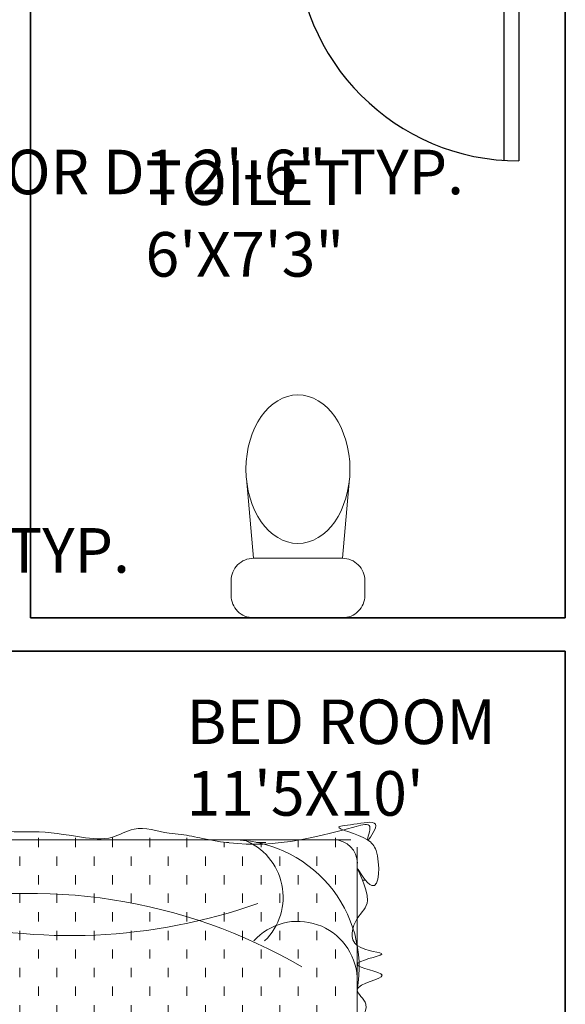
# Model space of a CAD drawing. Units: inches. Extents: x -26 to 575, y -18 to 513.
# Tile 9 of 28: x 196 to 269, y 191 to 324. Entities that reach past the tile are written whole.
import ezdxf

# ---------------------------------------------------------------- set-up
doc = ezdxf.new("R2010")
doc.units = ezdxf.units.IN
doc.header["$MEASUREMENT"] = 0
for name, color, linetype, lineweight in [('A-ANNO-DIMS', 2, 'Continuous', 18), ('A-AREA-IDEN', 7, 'Continuous', 18), ('A-DOOR', 3, 'Continuous', 25), ('A-FLOR-FIXT', 9, 'Continuous', 18), ('A-WALL', 7, 'Continuous', 35), ('Furniture', 8, 'Continuous', 15)]:
    doc.layers.add(name, color=color, linetype=linetype, lineweight=lineweight)
doc.styles.get("Standard").update_dxf_attribs({"font": 'arial.ttf', "height": 6})
doc.dimstyles.get("Standard").update_dxf_attribs({"dimtxt": 6, "dimasz": 0.18, "dimexe": 0.18, "dimexo": 0.0625, "dimgap": 0.09, "dimtad": 0, "dimtih": 1, "dimtoh": 1, "dimzin": 0, "dimdsep": 46, "dimlunit": 3, "dimtxsty": 'Standard', "dimcen": 0.09, "dimadec": 0, "dimazin": 0, "dimtfac": 1, "dimtofl": 0, "dimtmove": 0, "dimatfit": 3, "dimfxl": 1, "dimtolj": 1, "dimtzin": 0, "dimarcsym": 0})

# ---------------------------------------------------------------- blocks, each defined once
blk = doc.blocks.new('BED-DOUBLE-WITH-NIGHTSTANDS')
for p, q in [((1.93, 83.36), (1.93, 62.76)), ((21.61, 63.03), (21.61, 82.46)), ((22.83, 60.83), (22.83, 82.62)), ((81.88, 82.34), (81.88, 56.23)), ((82.67, 83.36), (82.67, 62.76)), ((102.35, 63.03), (102.35, 82.46)), ((23.23, 81.08), (0, 81.08)), ((10.27, 81.76), (8.94, 70.83)), ((21.24, 81.17), (81.88, 81.17)), ((103.97, 81.08), (80.74, 81.08)), ((20.89, 80.15), (2.67, 80.15)), ((2.67, 80.15), (2.67, 64.97)), ((20.89, 64.97), (20.89, 80.15)), ((82.67, 79.72), (21.06, 79.72)), ((101.63, 80.15), (83.41, 80.15)), ((83.41, 80.15), (83.41, 64.97)), ((101.63, 64.97), (101.63, 80.15)), ((92.57, 79.4), (92.57, 67.51)), ((14.67, 76.01), (4.51, 77.26)), ((44, 76.51), (44, 76.88)), ((46.83, 76.51), (46.83, 76.88)), ((8.06, 67.24), (12.03, 75.72)), ((12.03, 75.72), (14.23, 74.69)), ((25.06, 76.76), (22.83, 76.76)), ((41.17, 76.51), (40.96, 76.72)), ((41.17, 76.51), (41.43, 76.77)), ((41.17, 76.51), (41.17, 76.74)), ((56.23, 76.76), (41.36, 76.76)), ((44, 76.51), (43.73, 76.77)), ((44, 76.51), (44.26, 76.77)), ((46.83, 76.51), (46.56, 76.77)), ((46.83, 76.51), (47.09, 76.77)), ((57, 76.51), (56.74, 76.77)), ((57, 76.51), (57, 76.83)), ((57, 76.51), (57.27, 76.77)), ((81.88, 76.76), (59.39, 76.76)), ((59.83, 76.51), (59.59, 76.74)), ((59.83, 76.51), (59.83, 76.72)), ((59.83, 76.51), (60.02, 76.69)), ((11.46, 75.32), (8.12, 68.2)), ((14.23, 74.69), (10.26, 66.21)), ((11.77, 75.18), (11.46, 75.32)), ((25.61, 75.09), (25.35, 75.36)), ((25.61, 75.09), (25.61, 75.47)), ((25.61, 75.09), (25.88, 75.36)), ((28.44, 75.09), (28.18, 75.36)), ((28.44, 75.09), (28.44, 75.47)), ((28.44, 75.09), (28.71, 75.36)), ((31.27, 75.09), (31, 75.36)), ((31.27, 75.09), (31.27, 75.47)), ((31.27, 75.09), (31.53, 75.36)), ((34.1, 75.09), (33.83, 75.36)), ((34.1, 75.09), (34.1, 75.47)), ((34.1, 75.09), (34.36, 75.36)), ((36.93, 75.09), (36.66, 75.36)), ((36.93, 75.09), (36.93, 75.47)), ((36.93, 75.09), (37.19, 75.36)), ((39.75, 75.09), (39.49, 75.36)), ((39.75, 75.09), (39.75, 75.47)), ((39.75, 75.09), (40.02, 75.36)), ((42.58, 75.09), (42.32, 75.36)), ((42.58, 75.09), (42.58, 75.47)), ((42.58, 75.09), (42.85, 75.36)), ((45.41, 75.09), (45.15, 75.36)), ((45.41, 75.09), (45.41, 75.47)), ((45.41, 75.09), (45.68, 75.36)), ((48.24, 75.09), (47.97, 75.36)), ((48.24, 75.09), (48.24, 75.47)), ((48.24, 75.09), (48.5, 75.36)), ((51.07, 75.09), (50.8, 75.36)), ((51.07, 75.09), (51.07, 75.1)), ((51.07, 75.09), (51.07, 75.1)), ((53, 75.34), (53.03, 75.36)), ((55.59, 75.09), (55.32, 75.36)), ((55.59, 75.09), (55.59, 75.47)), ((55.59, 75.09), (55.85, 75.36)), ((58.42, 75.09), (58.15, 75.36)), ((58.42, 75.09), (58.42, 75.47)), ((58.42, 75.09), (58.68, 75.36)), ((61.25, 75.09), (60.98, 75.36)), ((61.25, 75.09), (61.25, 75.47)), ((61.25, 75.09), (61.51, 75.36)), ((64.07, 75.09), (63.81, 75.36)), ((64.07, 75.09), (64.07, 75.47)), ((64.07, 75.09), (64.34, 75.36)), ((66.9, 75.09), (66.64, 75.36)), ((66.9, 75.09), (66.9, 75.47)), ((66.9, 75.09), (67.17, 75.36)), ((69.73, 75.09), (69.47, 75.36)), ((69.73, 75.09), (69.73, 75.47)), ((69.73, 75.09), (70, 75.36)), ((72.56, 75.09), (72.29, 75.36)), ((72.56, 75.09), (72.56, 75.47)), ((72.56, 75.09), (72.82, 75.36)), ((75.39, 75.09), (75.12, 75.36)), ((75.39, 75.09), (75.39, 75.47)), ((75.39, 75.09), (75.65, 75.36)), ((78.22, 75.09), (77.95, 75.36)), ((78.22, 75.09), (78.22, 75.47)), ((78.22, 75.09), (78.48, 75.36)), ((13.24, 72.57), (11.03, 73.6)), ((14.13, 73), (11.6, 67.59)), ((19.14, 71.73), (13.98, 74.14)), ((17.98, 71.2), (14.13, 73)), ((27.03, 73.68), (26.76, 73.94)), ((27.03, 73.68), (27.03, 74.05)), ((27.03, 73.68), (27.29, 73.94)), ((29.85, 73.68), (29.59, 73.94)), ((29.85, 73.68), (30.12, 73.94)), ((29.86, 73.68), (29.86, 74.05)), ((32.68, 73.68), (32.42, 73.94)), ((32.68, 73.68), (32.68, 74.05)), ((32.68, 73.68), (32.95, 73.94)), ((35.51, 73.68), (35.25, 73.94)), ((35.51, 73.68), (35.51, 74.05)), ((35.51, 73.68), (35.78, 73.94)), ((38.34, 73.68), (38.07, 73.94)), ((38.34, 73.68), (38.34, 74.05)), ((38.34, 73.68), (38.61, 73.94)), ((41.17, 73.68), (40.9, 73.94)), ((41.17, 73.68), (41.17, 74.05)), ((41.17, 73.68), (41.43, 73.94)), ((44, 73.68), (43.73, 73.94)), ((44, 73.68), (44, 74.05)), ((44, 73.68), (44.26, 73.94)), ((46.83, 73.68), (46.56, 73.94)), ((46.83, 73.68), (46.83, 74.05)), ((46.83, 73.68), (47.09, 73.94)), ((49.65, 73.68), (49.39, 73.94)), ((49.65, 73.68), (49.65, 74.05)), ((49.65, 73.68), (49.92, 73.94)), ((54.17, 73.68), (53.91, 73.94)), ((54.17, 73.68), (54.17, 74.05)), ((54.17, 73.68), (54.44, 73.94)), ((57, 73.68), (56.74, 73.94)), ((57, 73.68), (57, 74.05)), ((57, 73.68), (57.27, 73.94)), ((59.83, 73.68), (59.57, 73.94)), ((59.83, 73.68), (59.83, 74.05)), ((59.83, 73.68), (60.1, 73.94)), ((62.66, 73.68), (62.39, 73.94)), ((62.66, 73.68), (62.66, 74.05)), ((62.66, 73.68), (62.92, 73.94)), ((65.49, 73.68), (65.22, 73.94)), ((65.49, 73.68), (65.49, 74.05)), ((65.49, 73.68), (65.75, 73.94)), ((68.32, 73.68), (68.05, 73.94)), ((68.32, 73.68), (68.32, 74.05)), ((68.32, 73.68), (68.58, 73.94)), ((71.14, 73.68), (70.88, 73.94)), ((71.14, 73.68), (71.41, 73.94)), ((71.15, 73.68), (71.15, 74.05)), ((73.97, 73.68), (73.71, 73.94)), ((73.97, 73.68), (73.97, 74.05)), ((73.97, 73.68), (74.24, 73.94)), ((76.8, 73.68), (76.54, 73.94)), ((76.8, 73.68), (76.8, 74.05)), ((76.8, 73.68), (77.07, 73.94)), ((79.63, 73.68), (79.36, 73.94)), ((79.63, 73.68), (79.63, 74.05)), ((79.63, 73.68), (79.9, 73.94)), ((98.47, 73.14), (86.67, 73.14)), ((15.8, 64.6), (19.14, 71.73)), ((25.61, 72.26), (25.35, 72.53)), ((25.61, 72.26), (25.61, 72.64)), ((25.61, 72.26), (25.88, 72.53)), ((28.44, 72.26), (28.18, 72.53)), ((28.44, 72.26), (28.44, 72.64)), ((28.44, 72.26), (28.71, 72.53)), ((31.27, 72.26), (31, 72.53)), ((31.27, 72.26), (31.27, 72.64)), ((31.27, 72.26), (31.53, 72.53)), ((34.1, 72.26), (33.83, 72.53)), ((34.1, 72.26), (34.1, 72.64)), ((34.1, 72.26), (34.36, 72.53)), ((36.93, 72.26), (36.66, 72.53)), ((36.93, 72.26), (36.93, 72.64)), ((36.93, 72.26), (37.19, 72.53)), ((39.75, 72.26), (39.49, 72.53)), ((39.75, 72.26), (39.75, 72.64)), ((39.75, 72.26), (40.02, 72.53)), ((42.58, 72.26), (42.32, 72.53)), ((42.58, 72.26), (42.58, 72.64)), ((42.58, 72.26), (42.85, 72.53)), ((45.41, 72.26), (45.15, 72.53)), ((45.41, 72.26), (45.41, 72.64)), ((45.41, 72.26), (45.68, 72.53)), ((48.24, 72.26), (47.97, 72.53)), ((48.24, 72.26), (48.24, 72.64)), ((48.24, 72.26), (48.5, 72.53)), ((55.59, 72.26), (55.32, 72.53)), ((55.59, 72.26), (55.59, 72.64)), ((55.59, 72.26), (55.85, 72.53)), ((58.42, 72.26), (58.15, 72.53)), ((58.42, 72.26), (58.42, 72.64)), ((58.42, 72.26), (58.68, 72.53)), ((61.25, 72.26), (60.98, 72.53)), ((61.25, 72.26), (61.25, 72.64)), ((61.25, 72.26), (61.51, 72.53)), ((64.07, 72.26), (63.81, 72.53)), ((64.07, 72.26), (64.07, 72.64)), ((64.07, 72.26), (64.34, 72.53)), ((66.9, 72.26), (66.64, 72.53)), ((66.9, 72.26), (66.9, 72.64)), ((66.9, 72.26), (67.17, 72.53)), ((69.73, 72.26), (69.47, 72.53)), ((69.73, 72.26), (69.73, 72.64)), ((69.73, 72.26), (70, 72.53)), ((72.56, 72.26), (72.29, 72.53)), ((72.56, 72.26), (72.56, 72.64)), ((72.56, 72.26), (72.82, 72.53)), ((75.39, 72.26), (75.12, 72.53)), ((75.39, 72.26), (75.39, 72.64)), ((75.39, 72.26), (75.65, 72.53)), ((78.22, 72.26), (77.95, 72.53)), ((78.22, 72.26), (78.22, 72.64)), ((78.22, 72.26), (78.48, 72.53)), ((15.45, 65.79), (17.98, 71.2)), ((24.2, 70.85), (23.97, 71.08)), ((24.2, 70.85), (24.2, 71.23)), ((24.2, 70.85), (24.46, 71.12)), ((27.03, 70.85), (26.76, 71.12)), ((27.03, 70.85), (27.03, 71.23)), ((27.03, 70.85), (27.29, 71.12)), ((29.85, 70.85), (29.59, 71.12)), ((29.85, 70.85), (30.12, 71.12)), ((29.86, 70.85), (29.86, 71.23)), ((32.68, 70.85), (32.42, 71.12)), ((32.68, 70.85), (32.68, 71.23)), ((32.68, 70.85), (32.95, 71.12)), ((35.51, 70.85), (35.25, 71.12)), ((35.51, 70.85), (35.51, 71.23)), ((35.51, 70.85), (35.78, 71.12)), ((38.34, 70.85), (38.07, 71.12)), ((38.34, 70.85), (38.34, 71.23)), ((38.34, 70.85), (38.61, 71.12)), ((41.17, 70.85), (40.9, 71.12)), ((41.17, 70.85), (41.17, 71.23)), ((41.17, 70.85), (41.43, 71.12)), ((44, 70.85), (43.73, 71.12)), ((44, 70.85), (44, 71.23)), ((44, 70.85), (44.26, 71.12)), ((46.83, 70.85), (46.56, 71.12)), ((46.83, 70.85), (46.83, 71.23)), ((46.83, 70.85), (47.09, 71.12)), ((49.65, 70.85), (49.39, 71.12)), ((49.65, 70.85), (49.65, 71.23)), ((49.65, 70.85), (49.92, 71.12)), ((54.17, 70.85), (53.91, 71.12)), ((54.17, 70.85), (54.17, 71.23)), ((54.17, 70.85), (54.44, 71.12)), ((57, 70.85), (56.74, 71.12)), ((57, 70.85), (57, 71.23)), ((57, 70.85), (57.27, 71.12)), ((59.83, 70.85), (59.57, 71.12)), ((59.83, 70.85), (59.83, 71.23)), ((59.83, 70.85), (60.1, 71.12)), ((62.66, 70.85), (62.39, 71.12)), ((62.66, 70.85), (62.66, 71.23)), ((62.66, 70.85), (62.92, 71.12)), ((65.49, 70.85), (65.22, 71.12)), ((65.49, 70.85), (65.49, 71.23)), ((65.49, 70.85), (65.75, 71.12)), ((68.32, 70.85), (68.05, 71.12)), ((68.32, 70.85), (68.32, 71.23)), ((68.32, 70.85), (68.58, 71.12)), ((71.14, 70.85), (70.88, 71.12)), ((71.14, 70.85), (71.41, 71.12)), ((71.15, 70.85), (71.15, 71.23)), ((73.97, 70.85), (73.71, 71.12)), ((73.97, 70.85), (73.97, 71.23)), ((73.97, 70.85), (74.24, 71.12)), ((76.8, 70.85), (76.54, 71.12)), ((76.8, 70.85), (76.8, 71.23)), ((76.8, 70.85), (77.07, 71.12)), ((79.63, 70.85), (79.36, 71.12)), ((79.63, 70.85), (79.63, 71.23)), ((79.63, 70.85), (79.9, 71.12)), ((11.14, 68.07), (8.93, 69.1)), ((25.61, 69.44), (25.35, 69.7)), ((25.61, 69.44), (25.61, 69.81)), ((25.61, 69.44), (25.88, 69.7)), ((28.44, 69.44), (28.18, 69.7)), ((28.44, 69.44), (28.44, 69.81)), ((28.44, 69.44), (28.71, 69.7)), ((31.27, 69.44), (31, 69.7)), ((31.27, 69.44), (31.27, 69.81)), ((31.27, 69.44), (31.53, 69.7)), ((34.1, 69.44), (33.83, 69.7)), ((34.1, 69.44), (34.1, 69.81)), ((34.1, 69.44), (34.36, 69.7)), ((36.93, 69.44), (36.66, 69.7)), ((36.93, 69.44), (36.93, 69.81)), ((36.93, 69.44), (37.19, 69.7)), ((39.75, 69.44), (39.49, 69.7)), ((39.75, 69.44), (39.75, 69.81)), ((39.75, 69.44), (40.02, 69.7)), ((42.58, 69.44), (42.32, 69.7)), ((42.58, 69.44), (42.58, 69.81)), ((42.58, 69.44), (42.85, 69.7)), ((45.41, 69.44), (45.15, 69.7)), ((45.41, 69.44), (45.41, 69.81)), ((45.41, 69.44), (45.68, 69.7)), ((48.24, 69.44), (47.97, 69.7)), ((48.24, 69.44), (48.24, 69.81)), ((48.24, 69.44), (48.5, 69.7)), ((51.05, 69.45), (50.8, 69.7)), ((53.01, 69.68), (53.03, 69.7)), ((55.59, 69.44), (55.32, 69.7)), ((55.59, 69.44), (55.59, 69.81)), ((55.59, 69.44), (55.85, 69.7)), ((58.42, 69.44), (58.15, 69.7)), ((58.42, 69.44), (58.42, 69.81)), ((58.42, 69.44), (58.68, 69.7)), ((61.25, 69.44), (60.98, 69.7)), ((61.25, 69.44), (61.25, 69.81)), ((61.25, 69.44), (61.51, 69.7)), ((64.07, 69.44), (63.81, 69.7)), ((64.07, 69.44), (64.07, 69.81)), ((64.07, 69.44), (64.34, 69.7)), ((66.9, 69.44), (66.64, 69.7)), ((66.9, 69.44), (66.9, 69.81)), ((66.9, 69.44), (67.17, 69.7)), ((69.73, 69.44), (69.47, 69.7)), ((69.73, 69.44), (69.73, 69.81)), ((69.73, 69.44), (70, 69.7)), ((72.56, 69.44), (72.29, 69.7)), ((72.56, 69.44), (72.56, 69.81)), ((72.56, 69.44), (72.82, 69.7)), ((75.39, 69.44), (75.12, 69.7)), ((75.39, 69.44), (75.39, 69.81)), ((75.39, 69.44), (75.65, 69.7)), ((78.22, 69.44), (77.95, 69.7)), ((78.22, 69.44), (78.22, 69.81)), ((78.22, 69.44), (78.48, 69.7)), ((8.12, 68.2), (8.43, 68.05)), ((24.2, 68.02), (23.93, 68.29)), ((24.2, 68.02), (24.2, 68.4)), ((24.2, 68.02), (24.46, 68.29)), ((27.03, 68.02), (26.76, 68.29)), ((27.03, 68.02), (27.03, 68.4)), ((27.03, 68.02), (27.29, 68.29)), ((29.85, 68.02), (29.59, 68.29)), ((29.85, 68.02), (30.12, 68.29)), ((29.86, 68.02), (29.86, 68.4)), ((32.68, 68.02), (32.42, 68.29)), ((32.68, 68.02), (32.68, 68.4)), ((32.68, 68.02), (32.95, 68.29)), ((35.51, 68.02), (35.25, 68.29)), ((35.51, 68.02), (35.51, 68.4)), ((35.51, 68.02), (35.78, 68.29)), ((38.34, 68.02), (38.07, 68.29)), ((38.34, 68.02), (38.34, 68.4)), ((38.34, 68.02), (38.61, 68.29)), ((41.17, 68.02), (40.9, 68.29)), ((41.17, 68.02), (41.17, 68.4)), ((41.17, 68.02), (41.43, 68.29)), ((44, 68.02), (43.73, 68.29)), ((44, 68.02), (44, 68.4)), ((44, 68.02), (44.26, 68.29)), ((46.83, 68.02), (46.56, 68.29)), ((46.83, 68.02), (46.83, 68.4)), ((46.83, 68.02), (47.09, 68.29)), ((49.65, 68.02), (49.39, 68.29)), ((49.65, 68.02), (49.65, 68.4)), ((49.65, 68.02), (49.92, 68.29)), ((54.17, 68.02), (53.91, 68.29)), ((54.17, 68.02), (54.17, 68.4)), ((54.17, 68.02), (54.44, 68.29)), ((57, 68.02), (56.74, 68.29)), ((57, 68.02), (57, 68.4)), ((57, 68.02), (57.27, 68.29)), ((59.83, 68.02), (59.57, 68.29)), ((59.83, 68.02), (59.83, 68.4)), ((59.83, 68.02), (60.1, 68.29)), ((62.66, 68.02), (62.39, 68.29)), ((62.66, 68.02), (62.66, 68.4)), ((62.66, 68.02), (62.92, 68.29)), ((65.49, 68.02), (65.22, 68.29)), ((65.49, 68.02), (65.49, 68.4)), ((65.49, 68.02), (65.75, 68.29)), ((68.32, 68.02), (68.05, 68.29)), ((68.32, 68.02), (68.32, 68.4)), ((68.32, 68.02), (68.58, 68.29)), ((71.14, 68.02), (70.88, 68.29)), ((71.14, 68.02), (71.41, 68.29)), ((71.15, 68.02), (71.15, 68.4)), ((73.97, 68.02), (73.71, 68.29)), ((73.97, 68.02), (73.97, 68.4)), ((73.97, 68.02), (74.24, 68.29)), ((76.8, 68.02), (76.54, 68.29)), ((76.8, 68.02), (76.8, 68.4)), ((76.8, 68.02), (77.07, 68.29)), ((79.63, 68.02), (79.36, 68.29)), ((79.63, 68.02), (79.63, 68.4)), ((79.63, 68.02), (79.9, 68.29)), ((10.26, 66.21), (8.06, 67.24)), ((10.64, 67.02), (15.8, 64.6)), ((11.6, 67.59), (15.45, 65.79)), ((25.61, 66.61), (25.35, 66.87)), ((25.61, 66.61), (25.61, 66.98)), ((25.61, 66.61), (25.88, 66.87)), ((28.44, 66.61), (28.18, 66.87)), ((28.44, 66.61), (28.44, 66.98)), ((28.44, 66.61), (28.71, 66.87)), ((31.27, 66.61), (31, 66.87)), ((31.27, 66.61), (31.27, 66.98)), ((31.27, 66.61), (31.53, 66.87)), ((34.1, 66.61), (33.83, 66.87)), ((34.1, 66.61), (34.1, 66.98)), ((34.1, 66.61), (34.36, 66.87)), ((36.93, 66.61), (36.66, 66.87)), ((36.93, 66.61), (36.93, 66.98)), ((36.93, 66.61), (37.19, 66.87)), ((39.75, 66.61), (39.49, 66.87)), ((39.75, 66.61), (39.75, 66.98)), ((39.75, 66.61), (40.02, 66.87)), ((42.58, 66.61), (42.32, 66.87)), ((42.58, 66.61), (42.58, 66.98)), ((42.58, 66.61), (42.85, 66.87)), ((45.41, 66.61), (45.15, 66.87)), ((45.41, 66.61), (45.41, 66.98)), ((45.41, 66.61), (45.68, 66.87)), ((48.24, 66.61), (47.97, 66.87)), ((48.24, 66.61), (48.24, 66.98)), ((48.24, 66.61), (48.5, 66.87)), ((51.07, 66.61), (50.8, 66.87)), ((51.07, 66.61), (51.07, 66.98)), ((51.07, 66.61), (51.33, 66.87)), ((52.76, 66.61), (52.49, 66.87)), ((52.76, 66.61), (52.76, 66.98)), ((52.76, 66.61), (53.03, 66.87)), ((55.59, 66.61), (55.32, 66.87)), ((55.59, 66.61), (55.59, 66.98)), ((55.59, 66.61), (55.85, 66.87)), ((58.42, 66.61), (58.15, 66.87)), ((58.42, 66.61), (58.42, 66.98)), ((58.42, 66.61), (58.68, 66.87)), ((61.25, 66.61), (60.98, 66.87)), ((61.25, 66.61), (61.25, 66.98)), ((61.25, 66.61), (61.51, 66.87)), ((64.07, 66.61), (63.81, 66.87)), ((64.07, 66.61), (64.07, 66.98)), ((64.07, 66.61), (64.34, 66.87)), ((66.9, 66.61), (66.64, 66.87)), ((66.9, 66.61), (66.9, 66.98)), ((66.9, 66.61), (67.17, 66.87)), ((69.73, 66.61), (69.47, 66.87)), ((69.73, 66.61), (69.73, 66.98)), ((69.73, 66.61), (70, 66.87)), ((72.56, 66.61), (72.29, 66.87)), ((72.56, 66.61), (72.56, 66.98)), ((72.56, 66.61), (72.82, 66.87)), ((75.39, 66.61), (75.12, 66.87)), ((75.39, 66.61), (75.39, 66.98)), ((75.39, 66.61), (75.65, 66.87)), ((78.22, 66.61), (77.95, 66.87)), ((78.22, 66.61), (78.22, 66.98)), ((78.22, 66.61), (78.48, 66.87)), ((81.04, 66.61), (80.78, 66.87)), ((81.04, 66.61), (81.04, 66.98)), ((81.04, 66.61), (81.25, 66.82)), ((2.67, 64.97), (20.89, 64.97)), ((24.2, 65.39), (24.2, 65.57)), ((24.29, 65.29), (24.46, 65.46)), ((27.03, 65.19), (26.76, 65.46)), ((27.03, 65.19), (27.03, 65.57)), ((27.03, 65.19), (27.29, 65.46)), ((29.85, 65.19), (29.59, 65.46)), ((29.85, 65.19), (30.12, 65.46)), ((29.86, 65.19), (29.86, 65.57)), ((32.68, 65.19), (32.42, 65.46)), ((32.68, 65.19), (32.68, 65.57)), ((32.68, 65.19), (32.95, 65.46)), ((35.33, 65.37), (35.25, 65.46)), ((35.51, 65.39), (35.51, 65.57)), ((35.74, 65.42), (35.78, 65.46)), ((46.77, 65.25), (46.56, 65.46)), ((46.83, 65.23), (46.83, 65.57)), ((46.86, 65.22), (47.09, 65.46)), ((49.65, 65.19), (49.39, 65.46)), ((49.65, 65.19), (49.65, 65.57)), ((49.65, 65.19), (49.92, 65.46)), ((54.17, 65.19), (53.91, 65.46)), ((54.17, 65.19), (54.17, 65.57)), ((54.17, 65.19), (54.44, 65.46)), ((57, 65.19), (56.74, 65.46)), ((57, 65.19), (57, 65.57)), ((57, 65.19), (57.27, 65.46)), ((59.83, 65.19), (59.57, 65.46)), ((59.83, 65.19), (59.83, 65.57)), ((59.83, 65.19), (60.1, 65.46)), ((62.66, 65.52), (62.66, 65.57)), ((65.49, 65.48), (65.49, 65.57)), ((65.74, 65.45), (65.75, 65.46)), ((68.32, 65.19), (68.05, 65.46)), ((68.32, 65.19), (68.32, 65.57)), ((68.32, 65.19), (68.58, 65.46)), ((71.14, 65.19), (70.88, 65.46)), ((71.14, 65.19), (71.41, 65.46)), ((71.15, 65.19), (71.15, 65.57)), ((73.97, 65.19), (73.71, 65.46)), ((73.97, 65.19), (73.97, 65.57)), ((73.97, 65.19), (74.24, 65.46)), ((76.8, 65.19), (76.54, 65.46)), ((76.8, 65.19), (76.8, 65.57)), ((76.8, 65.19), (77.07, 65.46)), ((79.63, 65.19), (79.36, 65.46)), ((79.63, 65.19), (79.63, 65.57)), ((79.63, 65.19), (79.9, 65.46)), ((82.15, 61.74), (82.15, 65.42)), ((83.41, 64.97), (101.63, 64.97)), ((0.45, 64.15), (23.14, 64.15)), ((55.59, 64.12), (55.59, 64.15)), ((81.19, 64.15), (103.88, 64.15)), ((78.27, 59.67), (78.27, 60.15)), ((20.77, 58.21), (20.77, 58.42)), ((25.77, 57.17), (25.77, 58.42)), ((30.77, 57.17), (30.77, 58.42)), ((35.77, 57.17), (35.77, 58.41)), ((70.77, 57.17), (70.77, 58.42)), ((75.77, 57.17), (75.77, 58.42)), ((80.77, 57.17), (80.77, 58.42)), ((21.39, 57.79), (21.31, 57.79)), ((26.39, 57.79), (25.14, 57.79)), ((31.39, 57.79), (30.14, 57.79)), ((36.39, 57.79), (35.14, 57.79)), ((41.39, 57.79), (40.14, 57.79)), ((40.77, 57.17), (40.77, 57.97)), ((45.77, 57.17), (45.77, 57.64)), ((50.77, 57.17), (50.77, 57.46)), ((55.77, 57.17), (55.77, 57.48)), ((60.77, 57.17), (60.77, 57.74)), ((66.39, 57.79), (65.14, 57.79)), ((65.77, 57.17), (65.77, 58.21)), ((71.39, 57.79), (70.14, 57.79)), ((76.39, 57.79), (75.14, 57.79)), ((81.39, 57.79), (80.14, 57.79)), ((23.27, 54.64), (23.27, 55.76)), ((28.27, 54.67), (28.27, 55.92)), ((33.27, 54.67), (33.27, 55.92)), ((38.27, 54.67), (38.27, 55.92)), ((43.27, 54.67), (43.27, 55.92)), ((48.27, 54.67), (48.27, 55.92)), ((53.27, 54.67), (53.27, 55.92)), ((58.27, 54.67), (58.27, 55.92)), ((63.27, 54.67), (63.27, 55.92)), ((68.27, 54.67), (68.27, 55.92)), ((73.27, 54.67), (73.27, 55.92)), ((78.27, 54.67), (78.27, 55.92)), ((83.27, 54.67), (83.27, 55.92)), ((28.89, 55.29), (27.64, 55.29)), ((33.89, 55.29), (32.64, 55.29)), ((38.89, 55.29), (37.64, 55.29)), ((43.89, 55.29), (42.64, 55.29)), ((48.89, 55.29), (47.64, 55.29)), ((53.89, 55.29), (52.64, 55.29)), ((58.89, 55.29), (57.64, 55.29)), ((63.89, 55.29), (62.64, 55.29)), ((68.89, 55.29), (67.64, 55.29)), ((73.89, 55.29), (72.64, 55.29)), ((78.89, 55.29), (77.64, 55.29)), ((83.89, 55.29), (82.64, 55.29)), ((30.77, 52.17), (30.77, 53.42)), ((35.77, 52.17), (35.77, 53.42)), ((40.77, 52.17), (40.77, 53.42)), ((45.77, 52.17), (45.77, 53.42)), ((50.77, 52.17), (50.77, 53.42)), ((55.77, 52.17), (55.77, 53.42)), ((60.77, 52.17), (60.77, 53.42)), ((65.77, 52.17), (65.77, 53.42)), ((70.77, 52.17), (70.77, 53.42)), ((75.77, 52.17), (75.77, 53.42)), ((80.77, 52.17), (80.77, 53.42)), ((26.39, 52.79), (25.62, 52.79)), ((31.39, 52.79), (30.14, 52.79)), ((36.39, 52.79), (35.14, 52.79)), ((41.39, 52.79), (40.14, 52.79)), ((46.39, 52.79), (45.14, 52.79)), ((51.39, 52.79), (50.14, 52.79)), ((56.39, 52.79), (55.14, 52.79)), ((61.39, 52.79), (60.14, 52.79)), ((66.39, 52.79), (65.14, 52.79)), ((71.39, 52.79), (70.14, 52.79)), ((76.39, 52.79), (75.14, 52.79)), ((81.39, 52.79), (80.14, 52.79)), ((23.27, 49.67), (23.27, 50.92)), ((28.27, 49.67), (28.27, 50.92)), ((33.27, 49.67), (33.27, 50.92)), ((38.27, 49.67), (38.27, 50.92)), ((43.27, 49.67), (43.27, 50.92)), ((48.27, 49.67), (48.27, 50.92)), ((53.27, 49.67), (53.27, 50.92)), ((58.27, 49.67), (58.27, 50.92)), ((63.27, 49.67), (63.27, 50.92)), ((68.27, 49.67), (68.27, 50.92)), ((73.27, 49.67), (73.27, 50.92)), ((78.27, 49.67), (78.27, 50.92)), ((83.27, 49.67), (83.27, 50.92)), ((23.89, 50.29), (22.64, 50.29)), ((28.89, 50.29), (27.64, 50.29)), ((33.89, 50.29), (32.64, 50.29)), ((38.89, 50.29), (37.64, 50.29)), ((43.89, 50.29), (42.64, 50.29)), ((48.89, 50.29), (47.64, 50.29)), ((53.89, 50.29), (52.64, 50.29)), ((58.89, 50.29), (57.64, 50.29)), ((63.89, 50.29), (62.64, 50.29)), ((68.89, 50.29), (67.64, 50.29)), ((73.89, 50.29), (72.64, 50.29)), ((78.89, 50.29), (77.64, 50.29)), ((83.89, 50.29), (82.64, 50.29)), ((21.39, 47.79), (20.41, 47.79)), ((20.77, 47.17), (20.77, 48.42)), ((26.39, 47.79), (25.14, 47.79)), ((31.39, 47.79), (30.14, 47.79)), ((30.77, 47.17), (30.77, 48.42)), ((36.39, 47.79), (35.14, 47.79)), ((35.77, 47.17), (35.77, 48.42)), ((41.39, 47.79), (40.14, 47.79)), ((40.77, 47.17), (40.77, 48.42)), ((46.39, 47.79), (45.14, 47.79)), ((45.77, 47.17), (45.77, 48.42)), ((51.39, 47.79), (50.14, 47.79)), ((50.77, 47.17), (50.77, 48.42)), ((56.39, 47.79), (55.14, 47.79)), ((55.77, 47.17), (55.77, 48.42)), ((66.39, 47.79), (65.14, 47.79)), ((65.77, 47.17), (65.77, 48.42)), ((71.39, 47.79), (70.14, 47.79)), ((70.77, 47.17), (70.77, 48.42)), ((76.39, 47.79), (75.14, 47.79)), ((75.77, 47.17), (75.77, 48.42)), ((81.39, 47.79), (80.14, 47.79)), ((80.77, 47.17), (80.77, 48.42)), ((23.89, 45.29), (22.64, 45.29)), ((23.27, 44.67), (23.27, 45.92)), ((28.89, 45.29), (27.64, 45.29)), ((28.27, 44.67), (28.27, 45.92)), ((33.89, 45.29), (32.64, 45.29)), ((33.27, 44.67), (33.27, 45.92)), ((38.89, 45.29), (37.64, 45.29)), ((38.27, 44.67), (38.27, 45.92)), ((43.89, 45.29), (42.64, 45.29)), ((43.27, 44.67), (43.27, 45.92)), ((48.89, 45.29), (47.64, 45.29)), ((48.27, 44.67), (48.27, 45.92)), ((53.89, 45.29), (52.64, 45.29)), ((53.27, 44.67), (53.27, 45.92)), ((58.89, 45.29), (57.64, 45.29)), ((63.89, 45.29), (62.64, 45.29)), ((63.27, 44.67), (63.27, 45.92)), ((68.89, 45.29), (67.64, 45.29)), ((68.27, 44.67), (68.27, 45.92)), ((73.89, 45.29), (72.64, 45.29)), ((73.27, 44.67), (73.27, 45.92)), ((78.89, 45.29), (77.64, 45.29)), ((78.27, 44.67), (78.27, 45.92)), ((83.89, 45.29), (82.64, 45.29)), ((83.27, 44.67), (83.27, 45.92)), ((21.39, 42.79), (20.14, 42.79)), ((20.77, 42.17), (20.77, 43.42)), ((26.39, 42.79), (25.14, 42.79)), ((31.39, 42.79), (30.14, 42.79)), ((30.77, 42.17), (30.77, 43.42)), ((36.39, 42.79), (35.14, 42.79)), ((35.77, 42.17), (35.77, 43.42)), ((41.39, 42.79), (40.14, 42.79)), ((40.77, 42.17), (40.77, 43.42)), ((46.39, 42.79), (45.14, 42.79)), ((45.77, 42.17), (45.77, 43.42)), ((51.39, 42.79), (50.14, 42.79)), ((50.77, 42.17), (50.77, 43.42)), ((56.39, 42.79), (55.14, 42.79)), ((55.77, 42.17), (55.77, 43.42)), ((61.39, 42.79), (60.14, 42.79)), ((66.09, 42.79), (65.14, 42.79)), ((65.77, 42.17), (65.77, 43.42)), ((70.77, 42.17), (70.77, 43.42)), ((71.78, 42.02), (71.78, 42.49)), ((75.77, 42.17), (75.77, 43.42)), ((76.39, 42.79), (76.07, 42.79)), ((81.39, 42.79), (80.14, 42.79)), ((80.77, 42.17), (80.77, 43.42)), ((86.39, 42.79), (85.14, 42.79)), ((85.77, 42.17), (85.77, 43.42)), ((70.3, 40.54), (70.3, 41.28)), ((72.15, 42.39), (71.41, 42.39)), ((73.26, 40.54), (73.26, 41.28)), ((76.21, 40.54), (76.21, 41.13)), ((81.88, 42.36), (81.88, 0)), ((18.89, 40.29), (17.83, 40.29)), ((18.27, 39.67), (18.27, 40.92)), ((23.89, 40.29), (22.64, 40.29)), ((23.27, 39.99), (23.27, 40.92)), ((28.89, 40.29), (27.64, 40.29)), ((28.27, 39.67), (28.27, 40.92)), ((33.89, 40.29), (32.64, 40.29)), ((33.27, 39.67), (33.27, 40.92)), ((38.89, 40.29), (37.64, 40.29)), ((38.27, 39.67), (38.27, 40.92)), ((43.89, 40.29), (42.64, 40.29)), ((43.27, 39.67), (43.27, 40.92)), ((48.89, 40.29), (47.64, 40.29)), ((48.27, 39.67), (48.27, 40.92)), ((53.89, 40.29), (52.64, 40.29)), ((53.27, 39.67), (53.27, 40.92)), ((58.89, 40.29), (57.64, 40.29)), ((62.9, 40.29), (62.64, 40.29)), ((63.27, 39.67), (63.27, 40.92)), ((65.87, 39.06), (65.87, 39.8)), ((67.35, 40.54), (67.35, 40.84)), ((67.72, 40.91), (67.48, 40.91)), ((68.27, 39.67), (68.27, 40.92)), ((68.83, 39.06), (68.83, 39.8)), ((70.67, 40.91), (69.93, 40.91)), ((71.78, 39.06), (71.78, 39.8)), ((73.62, 40.91), (72.89, 40.91)), ((73.27, 39.67), (73.27, 40.92)), ((74.73, 39.06), (74.73, 39.8)), ((76.58, 40.91), (75.84, 40.91)), ((77.68, 39.06), (77.68, 39.8)), ((78.27, 39.67), (78.27, 40.92)), ((83.89, 40.29), (82.64, 40.29)), ((83.27, 39.67), (83.27, 40.92)), ((22.83, 3.42), (22.83, 38.86)), ((66.24, 39.43), (65.5, 39.43)), ((69.2, 39.43), (68.46, 39.43)), ((72.15, 39.43), (71.41, 39.43)), ((75.1, 39.43), (74.36, 39.43)), ((78.05, 39.43), (77.32, 39.43)), ((25.77, 37.17), (25.77, 38.42)), ((30.77, 37.17), (30.77, 38.42)), ((35.77, 37.17), (35.77, 38.42)), ((40.77, 37.17), (40.77, 38.42)), ((45.77, 37.17), (45.77, 38.42)), ((50.77, 37.17), (50.77, 38.42)), ((55.77, 37.17), (55.77, 38.42)), ((61.39, 37.79), (60.14, 37.79)), ((60.77, 37.17), (60.77, 38.42)), ((64.77, 37.96), (64.03, 37.96)), ((64.4, 37.59), (64.4, 38.33)), ((66.39, 37.79), (65.14, 37.79)), ((65.77, 37.17), (65.77, 38.42)), ((67.72, 37.96), (66.98, 37.96)), ((67.35, 37.59), (67.35, 38.33)), ((70.67, 37.96), (69.93, 37.96)), ((71.39, 37.79), (70.14, 37.79)), ((70.3, 37.59), (70.3, 38.33)), ((70.77, 37.17), (70.77, 38.42)), ((73.62, 37.96), (72.89, 37.96)), ((73.26, 37.59), (73.26, 38.33)), ((76.39, 37.79), (75.14, 37.79)), ((75.77, 37.17), (75.77, 38.42)), ((76.45, 37.96), (75.84, 37.96)), ((76.21, 37.8), (76.21, 38.33)), ((81.39, 37.79), (80.14, 37.79)), ((80.77, 37.17), (80.77, 38.42)), ((28.27, 34.67), (28.27, 35.92)), ((33.27, 34.67), (33.27, 35.92)), ((38.27, 34.67), (38.27, 35.92)), ((43.27, 34.67), (43.27, 35.92)), ((48.27, 34.67), (48.27, 35.92)), ((53.27, 34.67), (53.27, 35.92)), ((58.27, 34.67), (58.27, 35.92)), ((59.97, 36.11), (59.97, 36.16)), ((63.29, 36.48), (62.55, 36.48)), ((62.92, 36.11), (62.92, 36.85)), ((63.27, 34.67), (63.27, 35.92)), ((66.24, 36.48), (65.5, 36.48)), ((65.87, 36.11), (65.87, 36.85)), ((68.27, 34.67), (68.27, 35.92)), ((69.2, 36.48), (68.46, 36.48)), ((68.83, 36.11), (68.83, 36.85)), ((72.15, 36.48), (71.41, 36.48)), ((71.78, 36.11), (71.78, 36.85)), ((73.27, 34.67), (73.27, 35.92)), ((74.53, 36.48), (74.36, 36.48)), ((74.73, 36.66), (74.73, 36.85)), ((78.27, 34.67), (78.27, 35.92)), ((17.66, 35.29), (17.64, 35.29)), ((58.89, 35.29), (57.64, 35.29)), ((58.86, 35), (58.12, 35)), ((58.49, 34.64), (58.49, 35.37)), ((61.81, 35), (61.08, 35)), ((61.44, 34.64), (61.44, 35.37)), ((63.89, 35.29), (62.64, 35.29)), ((64.77, 35), (64.03, 35)), ((64.4, 34.64), (64.4, 35.37)), ((67.72, 35), (66.98, 35)), ((67.35, 34.64), (67.35, 35.37)), ((68.89, 35.29), (67.64, 35.29)), ((70.67, 35), (69.93, 35)), ((70.3, 34.64), (70.3, 35.37)), ((73.89, 35.29), (72.64, 35.29)), ((73.01, 35), (72.89, 35)), ((73.26, 35.25), (73.26, 35.37)), ((78.89, 35.29), (77.64, 35.29)), ((25.77, 32.17), (25.77, 33.42)), ((30.77, 32.17), (30.77, 33.42)), ((35.77, 32.17), (35.77, 33.42)), ((40.77, 32.17), (40.77, 33.42)), ((45.77, 32.17), (45.77, 33.42)), ((50.77, 32.17), (50.77, 33.42)), ((51.11, 33.25), (51.11, 33.48)), ((54.43, 33.53), (53.69, 33.53)), ((54.06, 33.16), (54.06, 33.9)), ((55.77, 32.17), (55.77, 33.42)), ((57.38, 33.53), (56.65, 33.53)), ((57.02, 33.16), (57.02, 33.9)), ((60.34, 33.53), (59.6, 33.53)), ((59.97, 33.16), (59.97, 33.9)), ((60.77, 32.17), (60.77, 33.42)), ((63.29, 33.53), (62.55, 33.53)), ((62.92, 33.16), (62.92, 33.9)), ((66.24, 33.53), (65.5, 33.53)), ((65.77, 32.17), (65.77, 33.42)), ((65.87, 33.16), (65.87, 33.9)), ((69.2, 33.53), (68.46, 33.53)), ((68.83, 33.16), (68.83, 33.9)), ((70.77, 32.17), (70.77, 33.42)), ((71.47, 33.53), (71.41, 33.53)), ((71.78, 33.81), (71.78, 33.9)), ((75.77, 32.17), (75.77, 33.42)), ((80.77, 32.17), (80.77, 33.42)), ((55.54, 32.37), (55.54, 32.42)), ((58.86, 32.05), (58.12, 32.05)), ((58.49, 31.74), (58.49, 32.42)), ((61.81, 32.05), (61.08, 32.05)), ((61.44, 31.68), (61.44, 32.42)), ((64.77, 32.05), (64.03, 32.05)), ((64.4, 31.68), (64.4, 32.42)), ((67.72, 32.05), (66.98, 32.05)), ((67.35, 31.68), (67.35, 32.42)), ((28.27, 29.67), (28.27, 30.92)), ((33.27, 29.67), (33.27, 30.92)), ((38.27, 29.67), (38.27, 30.92)), ((43.27, 29.67), (43.27, 30.92)), ((48.27, 29.67), (48.27, 30.92)), ((53.27, 29.67), (53.27, 30.92)), ((58.27, 29.67), (58.27, 30.92)), ((63.27, 29.67), (63.27, 30.92)), ((68.27, 29.67), (68.27, 30.92)), ((73.27, 29.67), (73.27, 30.92)), ((78.27, 29.67), (78.27, 30.92)), ((83.27, 29.67), (83.27, 30.11)), ((25.77, 27.17), (25.77, 28.42)), ((30.77, 27.17), (30.77, 28.42)), ((35.77, 27.17), (35.77, 28.42)), ((40.77, 27.17), (40.77, 28.42)), ((45.77, 27.17), (45.77, 28.42)), ((50.77, 27.17), (50.77, 28.42)), ((55.77, 27.17), (55.77, 28.42)), ((60.77, 27.17), (60.77, 28.42)), ((65.77, 27.17), (65.77, 28.42)), ((70.77, 27.17), (70.77, 28.42)), ((75.77, 27.17), (75.77, 28.42)), ((80.77, 27.17), (80.77, 28.42)), ((28.27, 24.67), (28.27, 25.92)), ((33.27, 24.67), (33.27, 25.92)), ((38.27, 24.67), (38.27, 25.92)), ((43.27, 24.67), (43.27, 25.92)), ((48.27, 24.67), (48.27, 25.92)), ((53.27, 24.67), (53.27, 25.92)), ((58.27, 24.67), (58.27, 25.92)), ((63.27, 24.67), (63.27, 25.92)), ((68.27, 24.67), (68.27, 25.92)), ((73.27, 24.67), (73.27, 25.92)), ((78.27, 24.67), (78.27, 25.92)), ((25.77, 22.17), (25.77, 23.42)), ((30.77, 22.17), (30.77, 23.42)), ((35.77, 22.17), (35.77, 23.42)), ((40.77, 22.17), (40.77, 23.42)), ((45.77, 22.17), (45.77, 23.42)), ((50.77, 22.17), (50.77, 23.42)), ((55.77, 22.17), (55.77, 23.42)), ((60.77, 22.17), (60.77, 23.42)), ((65.77, 22.17), (65.77, 23.42)), ((70.77, 22.17), (70.77, 23.42)), ((75.77, 22.17), (75.77, 23.42)), ((80.77, 22.17), (80.77, 23.42)), ((28.27, 19.67), (28.27, 20.92)), ((33.27, 19.67), (33.27, 20.92)), ((38.27, 19.67), (38.27, 20.92)), ((43.27, 19.67), (43.27, 20.92)), ((48.27, 19.67), (48.27, 20.92)), ((53.27, 19.67), (53.27, 20.92)), ((58.27, 19.67), (58.27, 20.92)), ((63.27, 19.67), (63.27, 20.92)), ((68.27, 19.67), (68.27, 20.92)), ((73.27, 19.67), (73.27, 20.92)), ((78.27, 19.67), (78.27, 20.92)), ((25.77, 17.17), (25.77, 18.42)), ((30.77, 17.17), (30.77, 18.42)), ((35.77, 17.17), (35.77, 18.42)), ((40.77, 17.17), (40.77, 18.42)), ((45.77, 17.17), (45.77, 18.42)), ((50.77, 17.17), (50.77, 18.42)), ((55.77, 17.17), (55.77, 18.42)), ((60.77, 17.17), (60.77, 18.42)), ((65.77, 17.17), (65.77, 18.42)), ((70.77, 17.17), (70.77, 18.42)), ((75.77, 17.17), (75.77, 18.42)), ((80.77, 17.17), (80.77, 18.42)), ((28.27, 14.67), (28.27, 15.92)), ((33.27, 14.67), (33.27, 15.92)), ((38.27, 14.67), (38.27, 15.92)), ((43.27, 14.67), (43.27, 15.92)), ((48.27, 14.67), (48.27, 15.92)), ((53.27, 14.67), (53.27, 15.92)), ((58.27, 14.67), (58.27, 15.92)), ((63.27, 14.67), (63.27, 15.92)), ((68.27, 14.67), (68.27, 15.92)), ((73.27, 14.67), (73.27, 15.92)), ((78.27, 14.67), (78.27, 15.92)), ((83.27, 15.26), (83.27, 15.92)), ((25.77, 12.17), (25.77, 13.42)), ((30.77, 12.17), (30.77, 13.42)), ((35.77, 12.17), (35.77, 13.42)), ((40.77, 12.17), (40.77, 13.42)), ((45.77, 12.17), (45.77, 13.42)), ((50.77, 12.17), (50.77, 13.42)), ((55.77, 12.17), (55.77, 13.42)), ((60.77, 12.17), (60.77, 13.42)), ((65.77, 12.17), (65.77, 13.42)), ((70.77, 12.17), (70.77, 13.42)), ((75.77, 12.17), (75.77, 13.42)), ((80.77, 12.17), (80.77, 13.42)), ((28.27, 9.67), (28.27, 10.92)), ((33.27, 9.67), (33.27, 10.92)), ((38.27, 9.67), (38.27, 10.92)), ((43.27, 9.67), (43.27, 10.92)), ((48.27, 9.67), (48.27, 10.92)), ((53.27, 9.67), (53.27, 10.92)), ((58.27, 9.67), (58.27, 10.92)), ((63.27, 9.67), (63.27, 10.92)), ((68.27, 9.67), (68.27, 10.92)), ((73.27, 9.67), (73.27, 10.92)), ((78.27, 9.67), (78.27, 10.92)), ((83.27, 9.67), (83.27, 10.2)), ((25.77, 7.17), (25.77, 8.42)), ((30.77, 7.17), (30.77, 8.42)), ((35.77, 7.17), (35.77, 8.42)), ((40.77, 7.17), (40.77, 8.42)), ((45.77, 7.17), (45.77, 8.42)), ((50.77, 7.17), (50.77, 8.42)), ((55.77, 7.17), (55.77, 8.42)), ((60.77, 7.17), (60.77, 8.42)), ((65.77, 7.17), (65.77, 8.42)), ((70.77, 7.17), (70.77, 8.42)), ((75.77, 7.17), (75.77, 8.42)), ((80.77, 7.17), (80.77, 8.42)), ((22.12, 7.87), (21.71, 7.87)), ((28.27, 4.67), (28.27, 5.92)), ((33.27, 4.67), (33.27, 5.92)), ((38.27, 4.67), (38.27, 5.92)), ((43.27, 4.67), (43.27, 5.92)), ((48.27, 4.67), (48.27, 5.92)), ((53.27, 4.67), (53.27, 5.92)), ((58.27, 4.67), (58.27, 5.92)), ((63.27, 4.67), (63.27, 5.92)), ((68.27, 4.67), (68.27, 5.92)), ((73.27, 4.67), (73.27, 5.92)), ((78.27, 4.67), (78.27, 5.92)), ((25.77, 2.17), (25.77, 3.42)), ((30.77, 2.46), (30.77, 3.42)), ((36.39, 2.79), (35.14, 2.79)), ((35.77, 3), (35.77, 3.42)), ((40.4, 2.79), (40.14, 2.79)), ((40.77, 2.75), (40.77, 3.42)), ((45.77, 2.17), (45.77, 3.42)), ((50.77, 2.17), (50.77, 3.42)), ((55.77, 2.17), (55.77, 3.42)), ((60.77, 2.17), (60.77, 3.42)), ((65.77, 2.17), (65.77, 3.42)), ((70.77, 2.17), (70.77, 3.42)), ((75.77, 2.41), (75.77, 3.42)), ((80.77, 2.17), (80.77, 3.42)), ((85.58, 2.43), (23.7, 2.43))]:
    blk.add_line(p, q)
for centre, radius in [((9.65, 76.68), 4.06), ((9.65, 76.68), 3.73), ((9.65, 76.68), 1.87), ((9.65, 76.68), 1.7), ((92.82, 73.14), 3.85), ((92.82, 73.14), 2.27), ((60.49, 47.37), 2.36), ((52.63, 28.52), 2.75)]:
    blk.add_circle(centre, radius)
for centre, radius, start, end in [((18.64, 72.67), 7.53, 354.3248, 27.7728), ((41.09, 50.38), 26, 95.0264, 117.3299), ((40.61, 70.41), 11.46, 327.7555, 34.1397), ((64.24, 66.16), 9.79, 78.7884, 122.5362), ((83.34, 72.35), 4.66, 124.7345, 186.5526), ((44.42, 57.1), 10.59, 48.8713, 93.3448), ((76.2, 84.7), 20.36, 248.1857, 275.9106), ((27.06, 44.47), 7.56, 311.0401, 36.1384), ((86.26, 43.42), 4.94, 128.8354, 178.0038), ((39.78, 19.64), 17.21, 170.0678, 270.9321), ((30.83, 21.41), 8.01, 183.5361, 317.8486), ((66.97, 82.6), 72.97, 239.8126, 282.5472), ((41.05, 10.13), 8.24, 134.2353, 249.0585), ((61.48, -60.53), 75.85, 75.7143, 109.4459), ((25.97, 5.58), 3.15, 180, 270), ((78.73, 5.58), 3.15, 270, 0)]:
    blk.add_arc(centre, radius, start, end)
for points, knots in [([(24.71, 64.66), (26.06, 64.63), (33, 64.48), (41.95, 67.2), (49.02, 64.48), (52.79, 64.86), (50.63, 69.88), (50.43, 72.76), (51.76, 76.03), (43.45, 78.05), (36.59, 75.07), (28.31, 76.39), (25.37, 76.36), (24.84, 76.35)], [0, 0, 0, 0, 4.049674, 20.880819, 25.932041, 26.821979, 31.217024, 36.043065, 37.533831, 40.150607, 55.448466, 62.672935, 64.278467, 64.278467, 64.278467, 64.278467]), ([(81.33, 64.66), (77.47, 64.34), (71.21, 63.83), (62.27, 66.78), (55.98, 62.89), (52.05, 65.92), (52.93, 69.57), (53.86, 72.57), (52.44, 75.93), (58.7, 77.69), (63.65, 75.45), (70.13, 76.24), (74.45, 76.62), (78.12, 76.32), (80.32, 76.35), (81.04, 76.35)], [0, 0, 0, 0, 11.502554, 18.635017, 27.654655, 28.800011, 32.595859, 36.914018, 38.927328, 41.544104, 52.009639, 56.262652, 60.661637, 65.075538, 67.252844, 67.252844, 67.252844, 67.252844]), ([(81.3, 78.04), (80.68, 75.31), (79.67, 70.85), (81.18, 67.62), (83.38, 62.52), (82.09, 64.57), (81.59, 64.66)], [0, 0, 0, 0, 7.603099, 12.404488, 14.892294, 16.432626, 16.432626, 16.432626, 16.432626]), ([(25.07, 76.86), (24.73, 74.84), (24.15, 71.41), (22.76, 66.41), (24.85, 64.9), (25.6, 63.75), (26.07, 63.83)], [0, 0, 0, 0, 6.47304, 11.006869, 12.799679, 14.2185, 14.2185, 14.2185, 14.2185]), ([(81.88, 65.42), (81.77, 63.58), (81.62, 61.27), (84.25, 59.71), (83.77, 58.74), (83.52, 58.22)], [0, 0, 0, 0, 4.973031, 6.254082, 7.747585, 7.747585, 7.747585, 7.747585]), ([(83.91, 58.07), (84.56, 56.74), (85.58, 54.64), (82.28, 53.65), (82.99, 50.72), (85.33, 50.53), (84.9, 48.23), (82.06, 47.25), (85.77, 45.87), (88.76, 44.17), (85.37, 42.03), (87.05, 39.3), (78.86, 37.34), (72.98, 51.01), (54.08, 29.24), (35.91, 32.92), (20.82, 41.99), (17.17, 32.57), (16.24, 37.8), (18.71, 38.79), (15.91, 43.44), (22.37, 43.45), (20.93, 46.18), (20.19, 47.95), (20.32, 52.93), (35.13, 52.6), (16.25, 58.94), (26.31, 59.48), (35.16, 58.38), (54.32, 56.67), (69.44, 58.46), (82.07, 60.88), (83.53, 58.65), (83.91, 58.07)], [0, 0, 0, 0, 3.481099, 5.475811, 8.043407, 9.436812, 11.330727, 12.888379, 16.258255, 18.252967, 21.734596, 23.018392, 26.087149, 38.445812, 54.5649, 86.600283, 92.594507, 98.286547, 100.905288, 101.70342, 105.471876, 109.954916, 110.954151, 113.598333, 116.114301, 124.231953, 133.25029, 137.509046, 143.991555, 164.906349, 189.961005, 195.579007, 197.573325, 197.573325, 197.573325, 197.573325]), ([(23.43, 55.19), (24.49, 55), (27.11, 54.54), (29.42, 53.18), (30.79, 52.36)], [0, 0, 0, 0, 3.194191, 7.94245, 7.94245, 7.94245, 7.94245]), ([(83.72, 54.2), (82.76, 53.38), (78.97, 50.14), (73.79, 50.03), (69.93, 49.96)], [0, 0, 0, 0, 3.737027, 14.742384, 14.742384, 14.742384, 14.742384]), ([(82.45, 38.63), (79.86, 38.49), (74.81, 38.21), (68.7, 28.86), (57.63, 32.1), (43.09, 34.7), (32.13, 32.98), (18.89, 30.82), (17.48, 34.15), (16.98, 35.35)], [0, 0, 0, 0, 7.385187, 14.402621, 29.694422, 35.583277, 59.348121, 65.733553, 69.320983, 69.320983, 69.320983, 69.320983]), ([(82.95, 38.85), (82.91, 38.17), (82.85, 36.97), (81.76, 35.43), (82.66, 33.92), (82.17, 32.16), (83.17, 30.81), (83.54, 28.6), (81.84, 26.13), (84.59, 22.62), (82.27, 21.86), (82.5, 20.48), (82.77, 18.98), (83.36, 17.21), (83.5, 15.41), (82.61, 14.09), (82.87, 12.46), (82.71, 11.04), (83.72, 9.61), (82.91, 7.55), (83.23, 5.58), (83.08, 3.39), (85.08, 3.34), (83.88, 2.36), (83.09, 3.04), (82.19, 1.93), (80.71, 0.69), (78.27, 1.05), (76.16, 2.63), (73.68, 2.58), (71.48, 0.95), (69.05, 1.47), (65.15, 1.19), (60.81, 2), (56.05, 2.59), (52.45, 0.27), (49.19, 1.51), (46.12, 1.7), (37.69, 3.67), (31.84, 3.18), (20.44, -0.09), (22.21, 3.75), (19.18, -0.44), (22.91, 0.39), (27.14, 0.63), (21.63, 1.85), (19.68, 4.27), (19.87, 11.16), (24.26, 3.84), (20.3, 10.76), (23.26, 12.85), (24.33, 17.43), (16.78, 17.59), (25.96, 19.23), (16.2, 20.68), (24.67, 22.01), (20.04, 24.96), (24.6, 28.15), (20.03, 29.6), (23.48, 31.6), (22.43, 34.55), (22.92, 41.18), (22.85, 37.06), (22.83, 35.35)], [0, 0, 0, 0, 2.033881, 3.581387, 5.07489, 6.704853, 8.655612, 9.757262, 13.24098, 16.903694, 18.063816, 18.788243, 20.635227, 22.875483, 24.324336, 25.871843, 27.320698, 29.140811, 29.950855, 32.312207, 34.847704, 36.565952, 37.541804, 38.447727, 39.194923, 40.100844, 41.912688, 45.194843, 46.251388, 49.875946, 51.496686, 54.215105, 56.7523, 63.316606, 67.484853, 70.581422, 75.324573, 76.965649, 79.915763, 100.671038, 102.483321, 104.317501, 106.523635, 109.038061, 111.571263, 115.809372, 117.667229, 122.411431, 125.445794, 129.976907, 132.758854, 136.424739, 139.918708, 143.481583, 147.135325, 151.002466, 153.252794, 157.23352, 159.244583, 161.905351, 164.097269, 169.015093, 172.531686, 172.531686, 172.531686, 172.531686])]:
    blk.add_open_spline(points, degree=3, knots=knots)
blk = doc.blocks.new('DOOR-SWING-30IN')
for p, q in [((-30, 0), (0, 0)), ((-2, 0), (-2, -30)), ((0, 0), (0, -30))]:
    blk.add_line(p, q)
blk.add_arc((0, 0), 30, 180, 270)
blk = doc.blocks.new('WC-FLOOR-MOUNT')
for p, q in [((-6, 8), (-6.95, 18.75)), ((6, 8), (6.95, 18.75))]:
    blk.add_line(p, q)
blk.add_lwpolyline([(-6, 8), (6, 8, -0.414214), (9, 5), (9, 3, -0.414214), (6, 0), (-6, 0, -0.414214), (-9, 3), (-9, 5, -0.414214)], format="xyb", close=True)
blk.add_ellipse((0, 20), major_axis=(0, 10), ratio=0.7)
blk = doc.blocks.new('*D16')
at = {"layer": 'A-ANNO-DIMS', "color": 0, "lineweight": -2, "transparency": 16777216}
for p, q in [((150.16, 298.57), (150.16, 303.19)), ((150.34, 303.01), (179.98, 303.01)), ((180.16, 298.57), (180.16, 303.19)), ((180.16, 303.01), (180.34, 303.01))]:
    blk.add_line(p, q, dxfattribs=at)
at = {"layer": 'A-ANNO-DIMS', "color": 0, "transparency": 16777216}
for points in [[(150.34, 303.04), (150.34, 302.98), (150.16, 303.01)], [(179.98, 303.04), (179.98, 302.98), (180.16, 303.01)]]:
    blk.add_solid(points, dxfattribs=at)
at = {"layer": 'Defpoints', "color": 0, "transparency": 16777216}
for p in [(180.16, 303.01), (150.16, 298.51), (180.16, 298.51)]:
    blk.add_point(p, dxfattribs=at)
at = {"layer": 'A-ANNO-DIMS', "color": 0, "transparency": 16777216, "insert": (218.82, 303.01), "char_height": 6, "attachment_point": 5}
blk.add_mtext('\\A1;DOOR D1 2\'-6" TYP.', dxfattribs=at)
blk = doc.blocks.new('*D24')
at = {"layer": 'A-ANNO-DIMS', "color": 0, "lineweight": -2, "transparency": 16777216}
for p, q in [((46.82, 261.72), (46.82, 251.9)), ((111.54, 261.72), (111.54, 251.9)), ((47, 252.08), (111.36, 252.08)), ((111.54, 252.08), (111.72, 252.08))]:
    blk.add_line(p, q, dxfattribs=at)
at = {"layer": 'A-ANNO-DIMS', "color": 0, "transparency": 16777216}
for points in [[(47, 252.11), (47, 252.05), (46.82, 252.08)], [(111.36, 252.11), (111.36, 252.05), (111.54, 252.08)]]:
    blk.add_solid(points, dxfattribs=at)
at = {"layer": 'Defpoints', "color": 0, "transparency": 16777216}
for p in [(46.82, 261.79), (111.54, 261.79), (111.54, 252.08)]:
    blk.add_point(p, dxfattribs=at)
at = {"layer": 'A-ANNO-DIMS', "color": 0, "transparency": 16777216, "insert": (162.09, 252.08), "char_height": 6, "attachment_point": 5}
blk.add_mtext('\\A1;DINING SET 5\'-4 1/2" TYP.', dxfattribs=at)

msp = doc.modelspace()

# ---------------------------------------------------------------- linework, layer by layer
at = {"layer": 'A-WALL'}
for p, q in [((197.177, 243.008), (197.177, 330.008)), ((269.177, 243.008), (269.177, 330.008)), ((269.177, 243.008), (197.177, 243.008)), ((269.177, 238.508), (138.677, 238.508)), ((269.177, 127.508), (269.177, 238.508))]:
    msp.add_line(p, q, dxfattribs=at)

# ---------------------------------------------------------------- block references
at = {"layer": 'A-DOOR'}
msp.add_blockref('DOOR-SWING-30IN', (262.921, 334.508), dxfattribs=at)
at = {"layer": 'A-FLOR-FIXT'}
msp.add_blockref('WC-FLOOR-MOUNT', (233.177, 243.008), dxfattribs=at)
at = {"layer": 'Furniture', "rotation": 180}
msp.add_blockref('BED-DOUBLE-WITH-NIGHTSTANDS', (263.993, 215.545), dxfattribs=at)

# ---------------------------------------------------------------- texts
at = {"layer": 'A-AREA-IDEN'}
for s, p in [('TOILET', (212.65, 298.563)), ('6\'X7\'3"', (212.65, 288.924)), ('BED ROOM', (218.169, 226.005)), ("11'5X10'", (218.169, 216.366))]:
    msp.add_text(s, height=6, rotation=0.00167, dxfattribs=at).set_placement(p)

# ---------------------------------------------------------------- dimensions: what is measured, and where the dimension line sits
at = {"layer": 'A-ANNO-DIMS'}
for base, p1, p2, text, picture, middle in [((180.159, 303.008), (150.159, 298.508), (180.159, 298.508), 'DOOR D1 <> TYP.', '*D16', (218.825, 303.008)), ((111.544, 252.079), (46.82, 261.787), (111.544, 261.787), 'DINING SET <> TYP.', '*D24', (162.09, 252.079))]:
    dim = msp.add_linear_dim(base=base, p1=p1, p2=p2, text=text, dimstyle='Standard', override={"dimdec": 1, "dimlfac": 1, "dimrnd": 0, "dimzin": 1, "dimdsep": 46, "dimlunit": 4, "dimfrac": 2}, dxfattribs=at)
    dim.commit()
    dim.dimension.update_dxf_attribs({"geometry": picture, "text_midpoint": middle})

doc.saveas('drawing.dxf')
